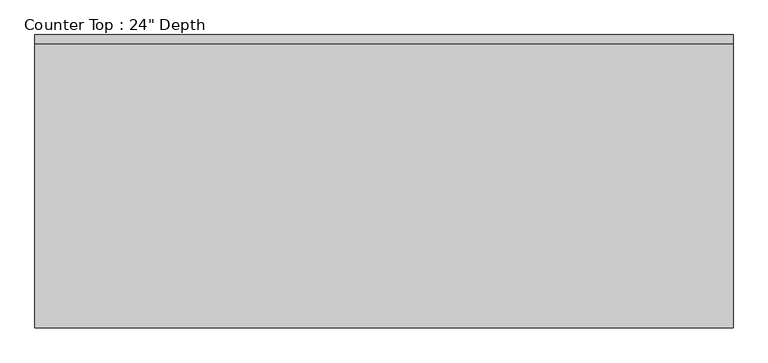
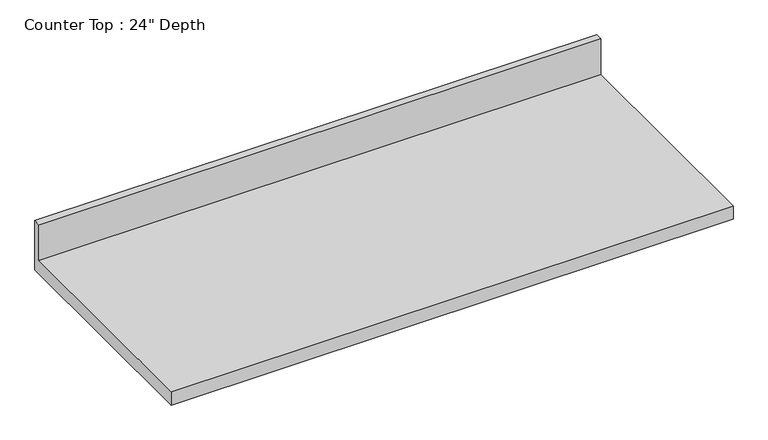
"""IFC4 building model written with IfcOpenShell, lengths in millimetres: furniture geometry."""

from ifc_helpers import new_model, si_unit, frame, origin, place, context, project, spatial, polyline, outline, extrude, source, transform, mapped, element, save


def furniture_9388d8e7(model_context):
    return source(origin(), model_context, "Body", "SweptSolid", [
        extrude(outline(polyline([(0.0, 1016.0), (0.0, 876.3), (-635.0, 876.3), (-635.0, 914.4), (-19.05, 914.4), (-19.05, 1016.0), (0.0, 1016.0)])), frame((-1200.4622951, 0.0, 0.0), z_axis=(1.0, 0.0, 0.0), x_axis=(0.0, 1.0, 0.0)), (0.0, 0.0, 1.0), 1511.3),
    ])


if __name__ == "__main__":
    model = new_model("IFC4")
    model_context = context("Model", 3, world=origin())
    ifc_project = project(units=[si_unit("LENGTHUNIT", "METRE", prefix="MILLI")], contexts=[model_context])
    site = spatial("IfcSite", under=ifc_project)
    building = spatial("IfcBuilding", under=site)
    placement = place(None, origin())
    furniture_shape = furniture_9388d8e7(model_context)
    element("IfcFurniture", 1, ObjectType="Counter Top : 24\" Depth", at=placement, inside=building, context=model_context, shape_type="MappedRepresentation", body=[
        mapped(furniture_shape, transform((0.0, 0.0, 0.0), x_axis=(1.0, 0.0, 0.0), y_axis=(0.0, 1.0, 0.0), z_axis=(0.0, 0.0, 1.0))),
    ])
    save(model, "model.ifc")

# Revit data of these elements
# Type "Counter Top : 24\" Depth"
#   Assembly Code = "C1030400"
#   Counter Thickness = 0' - 1 1/2"
#   Depth = 2' - 1"
#   Height = 3' - 0"
#   Length [instance default] = 8' - 0"
#   Counter Top Material = none
#   Default Elevation = 0
# Element 1 (IfcFurniture, "Counter Top : 24\" Depth")
#   Length = 4' - 11 1/2"
#   Materials on its faces: "Counter Top"
# Materials
#   "Counter Top": class "Wood", colour RGB 226 177 128, transparency 0
